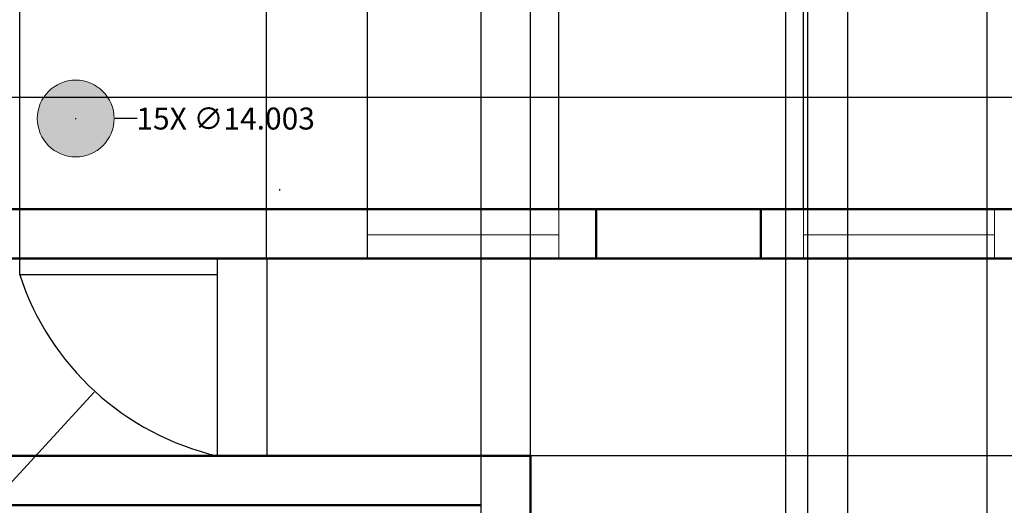
# Model space of a CAD drawing. Units: inches. Extents: x 1454 to 2136, y 626 to 1213.
# Tile 6 of 23: x 1561 to 1741, y 973 to 1062. Entities that reach past the tile are written whole.
import ezdxf

# ---------------------------------------------------------------- set-up
doc = ezdxf.new("R2010")
doc.units = ezdxf.units.IN
doc.header["$MEASUREMENT"] = 0
for name, color, linetype, lineweight in [('A-ANNO-DIMS', 2, 'Continuous', 18), ('A-DOOR', 3, 'Continuous', 25), ('A-FURN-PATT', 252, 'Continuous', 13), ('A-GLAZ', 4, 'Continuous', 18), ('A-PLNT-PATT', 116, 'Continuous', 13), ('A-WALL', 7, 'Continuous', 50), ('leafs', 112, 'Continuous', 18)]:
    doc.layers.add(name, color=color, linetype=linetype, lineweight=lineweight)
doc.styles.get("Standard").update_dxf_attribs({"font": 'arial.ttf'})
doc.dimstyles.get("Standard").update_dxf_attribs({"dimtxt": 4, "dimasz": 0.18, "dimexe": 0.18, "dimexo": 0.0625, "dimgap": 0.09, "dimtad": 0, "dimtih": 1, "dimtoh": 1, "dimdec": 0, "dimrnd": 6, "dimzin": 0, "dimdsep": 46, "dimlunit": 3, "dimtxsty": 'Standard', "dimcen": 0.09, "dimadec": 0, "dimazin": 0, "dimtfac": 1, "dimtdec": 0, "dimtofl": 0, "dimtmove": 0, "dimatfit": 3, "dimfxl": 1, "dimtolj": 1, "dimtzin": 0, "dimarcsym": 0})

# ---------------------------------------------------------------- blocks, each defined once
blk = doc.blocks.new('WIN-34_84')
blk.add_line((34.84, 4.31), (0, 4.31))
blk.add_lwpolyline([(34.84, 0), (0, 0), (0, 9), (34.84, 9)], close=True)
blk = doc.blocks.new('DOOR-LEAF-36')
blk.add_lwpolyline([(-36, 3), (0, 3), (0, 0), (-36, 0)], close=True)
blk = doc.blocks.new('*D33')
at = {"layer": 'A-ANNO-DIMS', "color": 0, "lineweight": -2, "transparency": 16777216}
for p, q in [((2032.49, 1126.28), (1462.37, 1126.28)), ((1462.55, 1126.1), (1462.55, 1056.38)), ((1462.55, 982.46), (1462.55, 1052.18)), ((2032.49, 982.28), (1462.37, 982.28))]:
    blk.add_line(p, q, dxfattribs=at)
at = {"layer": 'A-ANNO-DIMS', "color": 0, "transparency": 16777216}
for points in [[(1462.52, 1126.1), (1462.58, 1126.1), (1462.55, 1126.28)], [(1462.52, 982.46), (1462.58, 982.46), (1462.55, 982.28)]]:
    blk.add_solid(points, dxfattribs=at)
at = {"layer": 'Defpoints', "color": 0, "transparency": 16777216}
for p in [(1462.55, 1126.28), (2032.56, 1126.28), (2032.56, 982.28)]:
    blk.add_point(p, dxfattribs=at)
at = {"layer": 'A-ANNO-DIMS', "color": 0, "transparency": 16777216, "insert": (1462.55, 1054.28), "char_height": 4, "attachment_point": 5}
blk.add_mtext('\\A1;144', dxfattribs=at)
blk = doc.blocks.new('*D40')
at = {"layer": 'A-ANNO-DIMS', "color": 0, "lineweight": -2, "transparency": 16777216}
for p, q in [((1501.56, 877.34), (1501.56, 1210.46)), ((1501.74, 1210.28), (1569.24, 1210.28)), ((1645.38, 1210.28), (1577.87, 1210.28)), ((1645.56, 877.34), (1645.56, 1210.46))]:
    blk.add_line(p, q, dxfattribs=at)
at = {"layer": 'A-ANNO-DIMS', "color": 0, "transparency": 16777216}
for points in [[(1501.74, 1210.31), (1501.74, 1210.25), (1501.56, 1210.28)], [(1645.38, 1210.31), (1645.38, 1210.25), (1645.56, 1210.28)]]:
    blk.add_solid(points, dxfattribs=at)
at = {"layer": 'Defpoints', "color": 0, "transparency": 16777216}
for p in [(1645.56, 1210.28), (1501.56, 877.28), (1645.56, 877.28)]:
    blk.add_point(p, dxfattribs=at)
at = {"layer": 'A-ANNO-DIMS', "color": 0, "transparency": 16777216, "insert": (1573.56, 1210.28), "char_height": 4, "attachment_point": 5}
blk.add_mtext('\\A1;144', dxfattribs=at)
blk = doc.blocks.new('*D44')
at = {"layer": 'A-ANNO-DIMS', "color": 0, "lineweight": -2, "transparency": 16777216}
for p, q in [((1701.08, 909.11), (1701.08, 1210.46)), ((1701.26, 1210.28), (1784.96, 1210.28)), ((1885.07, 1210.28), (1801.37, 1210.28)), ((1885.25, 909.11), (1885.25, 1210.46))]:
    blk.add_line(p, q, dxfattribs=at)
at = {"layer": 'A-ANNO-DIMS', "color": 0, "transparency": 16777216}
for points in [[(1701.26, 1210.31), (1701.26, 1210.25), (1701.08, 1210.28)], [(1885.07, 1210.31), (1885.07, 1210.25), (1885.25, 1210.28)]]:
    blk.add_solid(points, dxfattribs=at)
at = {"layer": 'Defpoints', "color": 0, "transparency": 16777216}
for p in [(1885.25, 1210.28), (1701.08, 909.05), (1885.25, 909.05)]:
    blk.add_point(p, dxfattribs=at)
at = {"layer": 'A-ANNO-DIMS', "color": 0, "transparency": 16777216, "insert": (1793.16, 1210.28), "char_height": 4, "attachment_point": 5}
blk.add_mtext('\\A1;184.17', dxfattribs=at)
blk = doc.blocks.new('*D45')
at = {"layer": 'A-ANNO-DIMS', "color": 0, "lineweight": -2, "transparency": 16777216}
for p, q in [((1654.56, 913.34), (1654.56, 1210.46)), ((1654.74, 1210.28), (1670.92, 1210.28)), ((1700.9, 1210.28), (1684.72, 1210.28)), ((1701.08, 909.11), (1701.08, 1210.46))]:
    blk.add_line(p, q, dxfattribs=at)
at = {"layer": 'A-ANNO-DIMS', "color": 0, "transparency": 16777216}
for points in [[(1654.74, 1210.31), (1654.74, 1210.25), (1654.56, 1210.28)], [(1700.9, 1210.31), (1700.9, 1210.25), (1701.08, 1210.28)]]:
    blk.add_solid(points, dxfattribs=at)
at = {"layer": 'Defpoints', "color": 0, "transparency": 16777216}
for p in [(1701.08, 1210.28), (1654.56, 913.28), (1701.08, 909.05)]:
    blk.add_point(p, dxfattribs=at)
at = {"layer": 'A-ANNO-DIMS', "color": 0, "transparency": 16777216, "insert": (1677.82, 1210.28), "char_height": 4, "attachment_point": 5}
blk.add_mtext('\\A1;46.52', dxfattribs=at)
blk = doc.blocks.new('*D54')
at = {"layer": 'A-ANNO-DIMS', "color": 0, "lineweight": -2, "transparency": 16777216}
for p, q in [((1879.49, 1126.28), (1462.37, 1126.28)), ((1462.55, 1126.1), (1462.55, 1078.91)), ((1462.55, 1027.46), (1462.55, 1074.65)), ((1879.49, 1027.28), (1462.37, 1027.28))]:
    blk.add_line(p, q, dxfattribs=at)
at = {"layer": 'A-ANNO-DIMS', "color": 0, "transparency": 16777216}
for points in [[(1462.52, 1126.1), (1462.58, 1126.1), (1462.55, 1126.28)], [(1462.52, 1027.46), (1462.58, 1027.46), (1462.55, 1027.28)]]:
    blk.add_solid(points, dxfattribs=at)
at = {"layer": 'Defpoints', "color": 0, "transparency": 16777216}
for p in [(1879.56, 1126.28), (1462.55, 1027.28), (1879.56, 1027.28)]:
    blk.add_point(p, dxfattribs=at)
at = {"layer": 'A-ANNO-DIMS', "color": 0, "transparency": 16777216, "insert": (1462.55, 1076.78), "char_height": 4, "attachment_point": 5}
blk.add_mtext('\\A1;99', dxfattribs=at)
blk = doc.blocks.new('*D55')
at = {"layer": 'A-ANNO-DIMS', "color": 0, "lineweight": -2, "transparency": 16777216}
for p, q in [((1537.56, 1018.34), (1537.56, 1210.46)), ((1537.74, 1210.28), (1542.65, 1210.28)), ((1561.3, 1210.28), (1556.39, 1210.28)), ((1561.48, 1018.34), (1561.48, 1210.46))]:
    blk.add_line(p, q, dxfattribs=at)
at = {"layer": 'A-ANNO-DIMS', "color": 0, "transparency": 16777216}
for points in [[(1537.74, 1210.31), (1537.74, 1210.25), (1537.56, 1210.28)], [(1561.3, 1210.31), (1561.3, 1210.25), (1561.48, 1210.28)]]:
    blk.add_solid(points, dxfattribs=at)
at = {"layer": 'Defpoints', "color": 0, "transparency": 16777216}
for p in [(1561.48, 1210.28), (1537.56, 1018.28), (1561.48, 1018.28)]:
    blk.add_point(p, dxfattribs=at)
at = {"layer": 'A-ANNO-DIMS', "color": 0, "transparency": 16777216, "insert": (1549.52, 1210.28), "char_height": 4, "attachment_point": 5}
blk.add_mtext('\\A1;23.93', dxfattribs=at)
blk = doc.blocks.new('*D67')
at = {"layer": 'A-ANNO-DIMS', "color": 0, "lineweight": -2, "transparency": 16777216}
for p, q in [((1606.48, 1018.34), (1606.48, 1210.46)), ((1606.66, 1210.28), (1610.6, 1210.28)), ((1624.7, 1210.28), (1620.77, 1210.28)), ((1624.88, 1018.33), (1624.88, 1210.46))]:
    blk.add_line(p, q, dxfattribs=at)
at = {"layer": 'A-ANNO-DIMS', "color": 0, "transparency": 16777216}
for points in [[(1606.66, 1210.31), (1606.66, 1210.25), (1606.48, 1210.28)], [(1624.7, 1210.31), (1624.7, 1210.25), (1624.88, 1210.28)]]:
    blk.add_solid(points, dxfattribs=at)
at = {"layer": 'Defpoints', "color": 0, "transparency": 16777216}
for p in [(1624.88, 1210.28), (1606.48, 1018.28), (1624.88, 1018.27)]:
    blk.add_point(p, dxfattribs=at)
at = {"layer": 'A-ANNO-DIMS', "color": 0, "transparency": 16777216, "insert": (1615.68, 1210.28), "char_height": 4, "attachment_point": 5}
blk.add_mtext('\\A1;18.4', dxfattribs=at)
blk = doc.blocks.new('*D68')
at = {"layer": 'A-ANNO-DIMS', "color": 0, "lineweight": -2, "transparency": 16777216}
for p, q in [((1659.72, 1027.33), (1659.72, 1210.46)), ((1659.9, 1210.28), (1675.09, 1210.28)), ((1704.13, 1210.28), (1688.94, 1210.28)), ((1704.31, 1027.33), (1704.31, 1210.46))]:
    blk.add_line(p, q, dxfattribs=at)
at = {"layer": 'A-ANNO-DIMS', "color": 0, "transparency": 16777216}
for points in [[(1659.9, 1210.31), (1659.9, 1210.25), (1659.72, 1210.28)], [(1704.13, 1210.31), (1704.13, 1210.25), (1704.31, 1210.28)]]:
    blk.add_solid(points, dxfattribs=at)
at = {"layer": 'Defpoints', "color": 0, "transparency": 16777216}
for p in [(1704.31, 1210.28), (1659.72, 1027.27), (1704.31, 1027.27)]:
    blk.add_point(p, dxfattribs=at)
at = {"layer": 'A-ANNO-DIMS', "color": 0, "transparency": 16777216, "insert": (1682.02, 1210.28), "char_height": 4, "attachment_point": 5}
blk.add_mtext('\\A1;44.58', dxfattribs=at)
blk = doc.blocks.new('*D71')
at = {"layer": 'A-ANNO-DIMS', "color": 0, "lineweight": -2, "transparency": 16777216}
for p, q in [((1712.39, 694.26), (1712.39, 1210.46)), ((1712.57, 1210.28), (1718.61, 1210.28)), ((1737.62, 1210.28), (1731.58, 1210.28)), ((1737.8, 694.26), (1737.8, 1210.46))]:
    blk.add_line(p, q, dxfattribs=at)
at = {"layer": 'A-ANNO-DIMS', "color": 0, "transparency": 16777216}
for points in [[(1712.57, 1210.31), (1712.57, 1210.25), (1712.39, 1210.28)], [(1737.62, 1210.31), (1737.62, 1210.25), (1737.8, 1210.28)]]:
    blk.add_solid(points, dxfattribs=at)
at = {"layer": 'Defpoints', "color": 0, "transparency": 16777216}
for p in [(1737.8, 1210.28), (1712.39, 694.2), (1737.8, 694.2)]:
    blk.add_point(p, dxfattribs=at)
at = {"layer": 'A-ANNO-DIMS', "color": 0, "transparency": 16777216, "insert": (1725.09, 1210.28), "char_height": 4, "attachment_point": 5}
blk.add_mtext('\\A1;25.41', dxfattribs=at)
blk = doc.blocks.new('*D76')
at = {"layer": 'A-ANNO-DIMS', "color": 0, "lineweight": -2, "transparency": 16777216}
for p, q in [((1962.64, 1095.65), (1462.37, 1095.65)), ((1462.55, 1095.47), (1462.55, 1073.78)), ((1462.55, 1047.83), (1462.55, 1069.52)), ((1914.64, 1047.65), (1462.37, 1047.65))]:
    blk.add_line(p, q, dxfattribs=at)
at = {"layer": 'A-ANNO-DIMS', "color": 0, "transparency": 16777216}
for points in [[(1462.52, 1095.47), (1462.58, 1095.47), (1462.55, 1095.65)], [(1462.52, 1047.83), (1462.58, 1047.83), (1462.55, 1047.65)]]:
    blk.add_solid(points, dxfattribs=at)
at = {"layer": 'Defpoints', "color": 0, "transparency": 16777216}
for p in [(1962.71, 1095.65), (1462.55, 1047.65), (1914.71, 1047.65)]:
    blk.add_point(p, dxfattribs=at)
at = {"layer": 'A-ANNO-DIMS', "color": 0, "transparency": 16777216, "insert": (1462.55, 1071.65), "char_height": 4, "attachment_point": 5}
blk.add_mtext('\\A1;48', dxfattribs=at)
blk = doc.blocks.new('*D78')
at = {"layer": 'A-ANNO-DIMS', "color": 0, "lineweight": -2, "transparency": 16777216}
for p, q in [((1705.08, 833.11), (1705.08, 1210.46)), ((1705.26, 1210.28), (1726.04, 1210.28)), ((1752.9, 1210.28), (1732.12, 1210.28)), ((1753.08, 833.11), (1753.08, 1210.46))]:
    blk.add_line(p, q, dxfattribs=at)
at = {"layer": 'A-ANNO-DIMS', "color": 0, "transparency": 16777216}
for points in [[(1705.26, 1210.31), (1705.26, 1210.25), (1705.08, 1210.28)], [(1752.9, 1210.31), (1752.9, 1210.25), (1753.08, 1210.28)]]:
    blk.add_solid(points, dxfattribs=at)
at = {"layer": 'Defpoints', "color": 0, "transparency": 16777216}
for p in [(1753.08, 1210.28), (1705.08, 833.05), (1753.08, 833.05)]:
    blk.add_point(p, dxfattribs=at)
at = {"layer": 'A-ANNO-DIMS', "color": 0, "transparency": 16777216, "insert": (1729.08, 1210.28), "char_height": 4, "attachment_point": 5}
blk.add_mtext('\\A1;48', dxfattribs=at)
blk = doc.blocks.new('*D81')
at = {"layer": 'A-ANNO-DIMS', "color": 0, "lineweight": -2, "transparency": 16777216}
for p, q in [((1701.82, 1088.13), (1701.82, 1210.46)), ((1702, 1210.28), (1719.28, 1210.28)), ((1750.38, 1210.28), (1733.1, 1210.28)), ((1750.56, 1027.34), (1750.56, 1210.46))]:
    blk.add_line(p, q, dxfattribs=at)
at = {"layer": 'A-ANNO-DIMS', "color": 0, "transparency": 16777216}
for points in [[(1702, 1210.31), (1702, 1210.25), (1701.82, 1210.28)], [(1750.38, 1210.31), (1750.38, 1210.25), (1750.56, 1210.28)]]:
    blk.add_solid(points, dxfattribs=at)
at = {"layer": 'Defpoints', "color": 0, "transparency": 16777216}
for p in [(1701.82, 1210.28), (1701.82, 1088.07), (1750.56, 1027.28)]:
    blk.add_point(p, dxfattribs=at)
at = {"layer": 'A-ANNO-DIMS', "color": 0, "transparency": 16777216, "insert": (1726.19, 1210.28), "char_height": 4, "attachment_point": 5}
blk.add_mtext('\\A1;48.74', dxfattribs=at)
blk = doc.blocks.new('*D82')
at = {"layer": 'A-ANNO-DIMS', "color": 0, "lineweight": -2, "transparency": 16777216}
for p, q in [((1697.82, 1084.13), (1462.37, 1084.13)), ((1462.55, 1083.95), (1462.55, 1057.83)), ((1462.55, 1027.45), (1462.55, 1053.57)), ((1704.25, 1027.27), (1462.37, 1027.27))]:
    blk.add_line(p, q, dxfattribs=at)
at = {"layer": 'A-ANNO-DIMS', "color": 0, "transparency": 16777216}
for points in [[(1462.52, 1083.95), (1462.58, 1083.95), (1462.55, 1084.13)], [(1462.52, 1027.45), (1462.58, 1027.45), (1462.55, 1027.27)]]:
    blk.add_solid(points, dxfattribs=at)
at = {"layer": 'Defpoints', "color": 0, "transparency": 16777216}
for p in [(1462.55, 1084.13), (1697.88, 1084.13), (1704.31, 1027.27)]:
    blk.add_point(p, dxfattribs=at)
at = {"layer": 'A-ANNO-DIMS', "color": 0, "transparency": 16777216, "insert": (1462.55, 1055.7), "char_height": 4, "attachment_point": 5}
blk.add_mtext('\\A1;56.86', dxfattribs=at)
blk = doc.blocks.new('*D89')
at = {"layer": 'A-ANNO-DIMS', "color": 0, "lineweight": -2, "transparency": 16777216}
for p, q in [((1571.6, 1043.8), (1571.78, 1043.8)), ((1571.69, 1043.71), (1571.69, 1043.89)), ((1582.89, 1043.8), (1578.87, 1043.8))]:
    blk.add_line(p, q, dxfattribs=at)
at = {"layer": 'A-ANNO-DIMS', "color": 0, "transparency": 16777216}
blk.add_solid([(1578.87, 1043.83), (1578.87, 1043.77), (1578.69, 1043.8)], dxfattribs=at)
at = {"layer": 'Defpoints', "color": 0, "transparency": 16777216}
for p in [(1564.68, 1043.81), (1578.69, 1043.8)]:
    blk.add_point(p, dxfattribs=at)
at = {"layer": 'A-ANNO-DIMS', "color": 0, "transparency": 16777216, "insert": (1599.01, 1043.8), "char_height": 4, "attachment_point": 5}
blk.add_mtext('\\A1;15X ∅14.003', dxfattribs=at)
blk = doc.blocks.new('*D92')
at = {"layer": 'A-ANNO-DIMS', "color": 0, "lineweight": -2, "transparency": 16777216}
for p, q in [((1608.77, 1030.83), (1608.95, 1030.83)), ((1608.86, 1030.74), (1608.86, 1030.92)), ((1554.95, 972.02), (1575.05, 993.94)), ((1554.77, 972.02), (1554.95, 972.02))]:
    blk.add_line(p, q, dxfattribs=at)
at = {"layer": 'A-ANNO-DIMS', "color": 0, "transparency": 16777216}
blk.add_solid([(1575.02, 993.96), (1575.07, 993.92), (1575.17, 994.07)], dxfattribs=at)
at = {"layer": 'Defpoints', "color": 0, "transparency": 16777216}
for p in [(1608.86, 1030.83), (1575.17, 994.07)]:
    blk.add_point(p, dxfattribs=at)
at = {"layer": 'A-ANNO-DIMS', "color": 0, "transparency": 16777216, "insert": (1546.02, 972.02), "char_height": 4, "attachment_point": 5}
blk.add_mtext('\\A1;R49.86', dxfattribs=at)

msp = doc.modelspace()

# ---------------------------------------------------------------- hatches: boundary and pattern name
at = {"layer": 'A-FURN-PATT'}
h = msp.add_hatch(dxfattribs=at)
h.set_pattern_fill('ESCHER', color=256)
h.paths.add_polyline_path([(1511.3761, 923.7174, 1), (1525.379, 923.7174, 1)])
h.paths.add_polyline_path([(1525.379, 816.0542, 1), (1511.3761, 816.0542, 1)])
h.paths.add_polyline_path([(1525.379, 712.7345, 1), (1511.3761, 712.7345, 1)])
h.paths.add_polyline_path([(2070.5057, 794.3402, 1), (2056.5027, 794.3402, 1)])
h.paths.add_polyline_path([(2005.868, 1014.5578, 1), (1991.8651, 1014.5578, 1)])
h.paths.add_polyline_path([(1994.0647, 1066.7584, 1), (2008.0677, 1066.7584, 1)])
h.paths.add_polyline_path([(1919.5492, 1065.3848, 1), (1933.5521, 1065.3848, 1)])
h.paths.add_polyline_path([(1936.8517, 1013.7336, 1), (1922.8488, 1013.7336, 1)])
h.paths.add_polyline_path([(1824.6062, 1109.1557, 1), (1838.6091, 1109.1557, 1)])
at = {"layer": 'A-PLNT-PATT'}
h = msp.add_hatch(dxfattribs=at)
h.set_pattern_fill('ESCHER', color=256)
h.paths.add_polyline_path([(1767.2815, 694.0009, 1), (1753.2786, 694.0009, 1)])
h.paths.add_polyline_path([(1578.6873, 1043.8029, 1), (1564.6844, 1043.8029, 1)])

# ---------------------------------------------------------------- linework, layer by layer
at = {"layer": 'A-DOOR'}
for p, q in [((1606.4844, 1018.2825), (1606.4844, 982.2825)), ((1597.4844, 1015.2825), (1597.4844, 982.2825))]:
    msp.add_line(p, q, dxfattribs=at)
msp.add_arc((1608.86, 1030.8286), 49.8611, 198.167032, 256.812074, dxfattribs=at)
at = {"layer": 'A-WALL'}
for p, q in [((1750.5563, 1027.2825), (1546.5563, 1027.2825)), ((1666.5563, 1027.2825), (1666.5563, 1018.2825)), ((1696.5563, 1027.2825), (1696.5563, 1018.2825)), ((1714.5563, 1027.2825), (1714.5563, 1027.2667)), ((1843.5563, 1018.2825), (1537.5563, 1018.2825)), ((1654.5563, 982.2825), (1492.5563, 982.2825)), ((1654.5563, 982.2825), (1654.5563, 913.2825)), ((1645.5563, 973.2825), (1501.5563, 973.2825))]:
    msp.add_line(p, q, dxfattribs=at)
at = {"layer": 'leafs'}
msp.add_circle((1571.6859, 1043.8029), 7.0015, dxfattribs=at)

# ---------------------------------------------------------------- block references
at = {"layer": 'A-DOOR'}
msp.add_blockref('DOOR-LEAF-36', (1597.4844, 1015.2825), dxfattribs=at)
at = {"layer": 'A-GLAZ'}
for p in [(1624.8835, 1018.2667), (1704.308, 1018.2667)]:
    msp.add_blockref('WIN-34_84', p, dxfattribs=at)

# ---------------------------------------------------------------- dimensions: what is measured, and where the dimension line sits
at = {"layer": 'A-ANNO-DIMS'}
for base, p1, p2, override, picture, middle in [((1645.5563, 1210.2845), (1501.5563, 877.2825), (1645.5563, 877.2825), {"dimdec": 0, "dimlfac": 1, "dimrnd": 0, "dimzin": 0, "dimdsep": 46, "dimlunit": 2}, '*D40', (1573.5563, 1210.2845)), ((1561.4844, 1210.2845), (1537.5563, 1018.2825), (1561.4844, 1018.2825), {"dimdec": 2, "dimlfac": 1, "dimrnd": 0, "dimzin": 0, "dimdsep": 46, "dimlunit": 2}, '*D55', (1549.5203, 1210.2845)), ((1624.8835, 1210.2845), (1606.4844, 1018.2825), (1624.8835, 1018.2667), {"dimdec": 1, "dimlfac": 1, "dimrnd": 0, "dimzin": 0, "dimdsep": 46, "dimlunit": 2}, '*D67', (1615.6839, 1210.2845)), ((1701.0763, 1210.2845), (1654.5563, 913.2825), (1701.0763, 909.0476), {"dimdec": 2, "dimlfac": 1, "dimrnd": 0, "dimzin": 0, "dimdsep": 46, "dimlunit": 2}, '*D45', (1677.8163, 1210.2845)), ((1704.308, 1210.2845), (1659.7237, 1027.2667), (1704.308, 1027.2667), {"dimdec": 2, "dimlfac": 1, "dimrnd": 0, "dimzin": 0, "dimdsep": 46, "dimlunit": 2}, '*D68', (1682.0158, 1210.2845)), ((1885.2497, 1210.2845), (1701.0763, 909.0476), (1885.2497, 909.0476), {"dimdec": 2, "dimlfac": 1, "dimrnd": 0, "dimzin": 0, "dimdsep": 46, "dimlunit": 2}, '*D44', (1793.163, 1210.2845)), ((1701.8177, 1210.2845), (1750.5563, 1027.2825), (1701.8177, 1088.0655), {"dimdec": 2, "dimlfac": 1, "dimrnd": 0, "dimzin": 0, "dimdsep": 46, "dimlunit": 2}, '*D81', (1726.187, 1210.2845)), ((1753.0763, 1210.2845), (1705.0763, 833.0476), (1753.0763, 833.0476), {"dimdec": 0, "dimlfac": 1, "dimrnd": 0, "dimzin": 0, "dimdsep": 46, "dimlunit": 2}, '*D78', (1729.0763, 1210.2845)), ((1737.8001, 1210.2845), (1712.3887, 694.2005), (1737.8001, 694.2005), {"dimdec": 2, "dimlfac": 1, "dimrnd": 0, "dimzin": 0, "dimdsep": 46, "dimlunit": 2}, '*D71', (1725.0944, 1210.2845))]:
    dim = msp.add_linear_dim(base=base, p1=p1, p2=p2, dimstyle='Standard', override=override, dxfattribs=at)
    dim.commit()
    dim.dimension.update_dxf_attribs({"geometry": picture, "text_midpoint": middle})
for base, p1, p2, override, picture, middle in [((1462.5543, 1126.2825), (2032.5563, 982.2825), (2032.5563, 1126.2825), {"dimdec": 0, "dimlfac": 1, "dimrnd": 0, "dimzin": 0, "dimdsep": 46, "dimlunit": 2}, '*D33', (1462.5543, 1054.2825)), ((1462.5543, 1027.2825), (1879.5563, 1126.2825), (1879.5563, 1027.2825), {"dimdec": 0, "dimlfac": 1, "dimrnd": 0, "dimzin": 0, "dimdsep": 46, "dimlunit": 2}, '*D54', (1462.5543, 1076.7825)), ((1462.5543, 1047.6495), (1962.7068, 1095.6495), (1914.7068, 1047.6495), {"dimdec": 0, "dimlfac": 1, "dimrnd": 0, "dimzin": 0, "dimdsep": 46, "dimlunit": 2}, '*D76', (1462.5543, 1071.6495)), ((1462.5543, 1084.1285), (1704.308, 1027.2667), (1697.8807, 1084.1285), {"dimdec": 2, "dimlfac": 1, "dimrnd": 0, "dimzin": 0, "dimdsep": 46, "dimlunit": 2}, '*D82', (1462.5543, 1055.6976))]:
    dim = msp.add_linear_dim(base=base, p1=p1, p2=p2, angle=90, dimstyle='Standard', override=override, dxfattribs=at)
    dim.commit()
    dim.dimension.update_dxf_attribs({"geometry": picture, "text_midpoint": middle})
dim = msp.add_diameter_dim_2p(p1=(1564.6844, 1043.8059), p2=(1578.6873, 1043.8), text='15X <>', dimstyle='Standard', override={"dimdec": 3, "dimlfac": 1, "dimrnd": 0, "dimzin": 0, "dimdsep": 46, "dimlunit": 2}, dxfattribs=at)
dim.commit()
dim.dimension.update_dxf_attribs({"geometry": '*D89', "text_midpoint": (1582.8882, 1043.7982), "dimtype": 163})
dim = msp.add_radius_dim(center=(1608.86, 1030.8286), mpoint=(1575.1679, 994.0729), dimstyle='Standard', override={"dimdec": 2, "dimlfac": 1, "dimrnd": 0, "dimzin": 0, "dimdsep": 46, "dimlunit": 2}, dxfattribs=at)
dim.commit()
dim.dimension.update_dxf_attribs({"geometry": '*D92', "text_midpoint": (1546.0211, 972.0196), "dimtype": 164})

doc.saveas('drawing.dxf')
